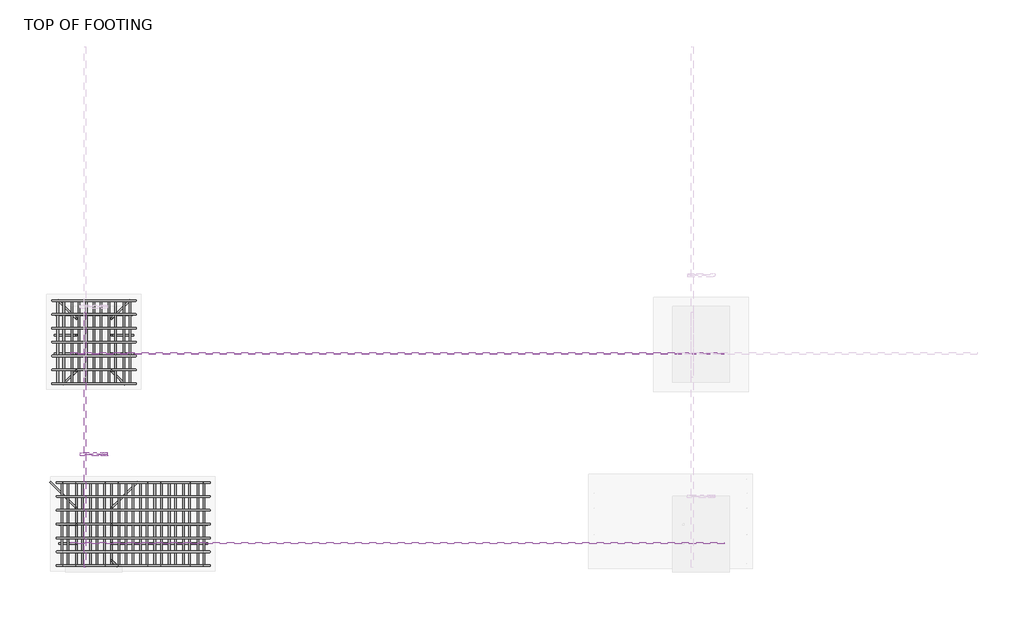
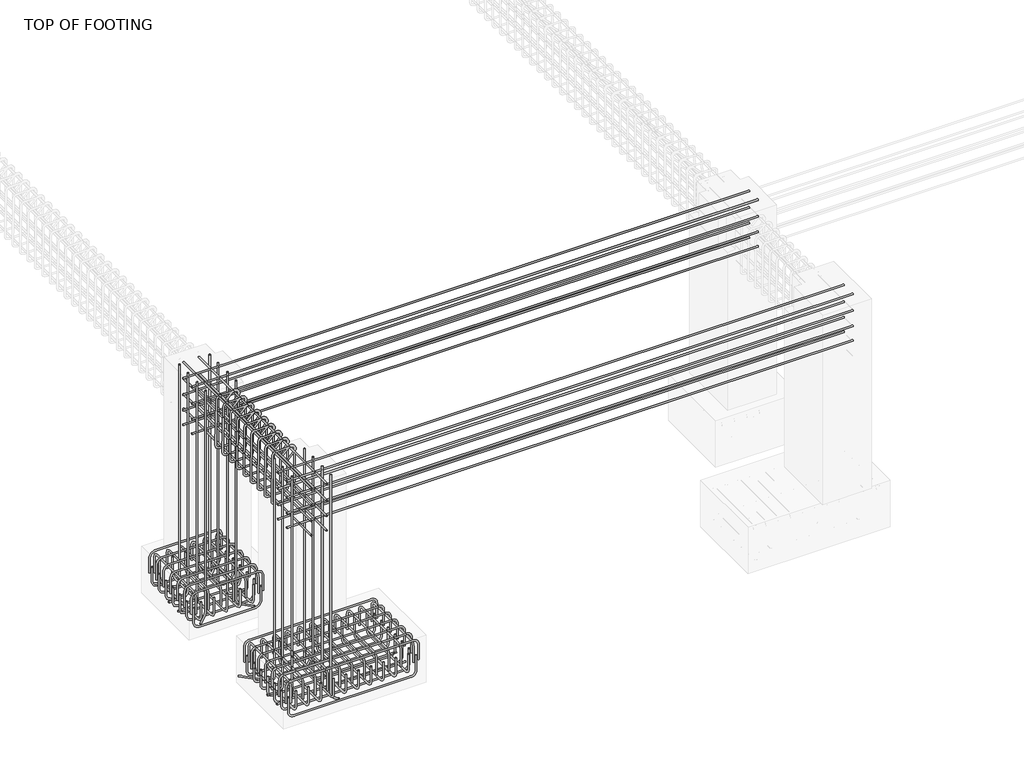
# One storey, part 2 of 8: 32 reinforcing bars.
"""IFC4 building model written with IfcOpenShell, lengths in millimetres."""

from ifc_helpers import new_model, si_unit, point, frame, origin, place, context, project, spatial, polyline, circle_curve, trimmed, segment, composite_curve, source, transform, mapped, element, save
from ifc_brep_helpers import swept_disk

model = new_model("IFC4")

# Units and contexts
model_context = context("Model", 3, world=origin())
ifc_project = project(units=[si_unit("LENGTHUNIT", "METRE", prefix="MILLI")], contexts=[model_context])

# Site, building, storey
site = spatial("IfcSite", under=ifc_project)
building = spatial("IfcBuilding", under=site)
storey = spatial("IfcBuildingStorey", under=building, Name="TOP OF FOOTING", Elevation=-1828.8)

# Reinforcing bars
placement = place(None, origin())
reinforcing_bar_shape = source(origin(), model_context, "Body", "SolidModel", [
    swept_disk(composite_curve([segment(polyline([(-6195.5877818, -134.3579757, -2021.245224), (-6195.5877818, -134.3579757, -2168.545224)]), True, "CONTINUOUS"), segment(trimmed(circle_curve(frame((-6241.9377818, -134.3579757, -2168.545224), z_axis=(0.0, 1.0, 0.0), x_axis=(46.350000000000364, 0.0, 0.0)), 46.35), [point((-6195.5877818, -134.3579757, -2168.545224))], [point((-6241.9377818, -134.3579757, -2214.895224))], True, "CARTESIAN"), True, "CONTINUOUS"), segment(polyline([(-6241.9377818, -134.3579757, -2214.895224), (-6762.8758647, -134.3579757, -2214.895224)]), True, "CONTINUOUS"), segment(trimmed(circle_curve(frame((-6762.8758647, -134.3579757, -2168.545224), z_axis=(0.0, 1.0, 0.0), x_axis=(0.0, 0.0, -46.34999999999991)), 46.35), [point((-6762.8758647, -134.3579757, -2214.895224))], [point((-6809.2258647, -134.3579757, -2168.545224))], True, "CARTESIAN"), True, "CONTINUOUS"), segment(polyline([(-6809.2258647, -134.3579757, -2168.545224), (-6809.2258647, -134.3579757, -2021.245224)]), True, "CONTINUOUS")], self_intersect=False), 6.35),
])
element("IfcReinforcingBar", 1, at=placement, inside=storey, context=model_context, shape_type="MappedRepresentation", body=[
    mapped(reinforcing_bar_shape, transform((0.0, 0.0, 0.0), x_axis=(1.0, 0.0, 0.0), y_axis=(0.0, 1.0, 0.0), z_axis=(0.0, 0.0, 1.0))),
    mapped(reinforcing_bar_shape, transform((0.0, -109.55, 0.0), x_axis=(1.0, 0.0, 0.0), y_axis=(0.0, 1.0, 0.0), z_axis=(0.0, 0.0, 1.0))),
    mapped(reinforcing_bar_shape, transform((0.0, -219.1, 0.0), x_axis=(1.0, 0.0, 0.0), y_axis=(0.0, 1.0, 0.0), z_axis=(0.0, 0.0, 1.0))),
    mapped(reinforcing_bar_shape, transform((0.0, -328.65, 0.0), x_axis=(1.0, 0.0, 0.0), y_axis=(0.0, 1.0, 0.0), z_axis=(0.0, 0.0, 1.0))),
    mapped(reinforcing_bar_shape, transform((0.0, -438.2, 0.0), x_axis=(1.0, 0.0, 0.0), y_axis=(0.0, 1.0, 0.0), z_axis=(0.0, 0.0, 1.0))),
    mapped(reinforcing_bar_shape, transform((0.0, -547.75, 0.0), x_axis=(1.0, 0.0, 0.0), y_axis=(0.0, 1.0, 0.0), z_axis=(0.0, 0.0, 1.0))),
    mapped(reinforcing_bar_shape, transform((0.0, -657.3, 0.0), x_axis=(1.0, 0.0, 0.0), y_axis=(0.0, 1.0, 0.0), z_axis=(0.0, 0.0, 1.0))),
])
reinforcing_bar_2_shape = source(origin(), model_context, "Body", "SolidModel", [
    swept_disk(composite_curve([segment(polyline([(-6831.1461367, -134.3579757, -2068.8), (-6831.1461367, -134.3579757, -1921.5)]), True, "CONTINUOUS"), segment(trimmed(circle_curve(frame((-6784.7961367, -134.3579757, -1921.5), z_axis=(0.0, 1.0, 0.0), x_axis=(-46.350000000000364, 0.0, 0.0)), 46.35), [point((-6831.1461367, -134.3579757, -1921.5))], [point((-6784.7961367, -134.3579757, -1875.15))], True, "CARTESIAN"), True, "CONTINUOUS"), segment(polyline([(-6784.7961367, -134.3579757, -1875.15), (-6220.1961367, -134.3579757, -1875.15)]), True, "CONTINUOUS"), segment(trimmed(circle_curve(frame((-6220.1961367, -134.3579757, -1921.5), z_axis=(0.0, 1.0, 0.0), x_axis=(0.0, 0.0, 46.34999999999991)), 46.35), [point((-6220.1961367, -134.3579757, -1875.15))], [point((-6173.8461367, -134.3579757, -1921.5))], True, "CARTESIAN"), True, "CONTINUOUS"), segment(polyline([(-6173.8461367, -134.3579757, -1921.5), (-6173.8461367, -134.3579757, -2068.8)]), True, "CONTINUOUS")], self_intersect=False), 6.35),
])
element("IfcReinforcingBar", 2, at=placement, inside=storey, context=model_context, shape_type="MappedRepresentation", body=[
    mapped(reinforcing_bar_2_shape, transform((0.0, 0.0, 0.0), x_axis=(1.0, 0.0, 0.0), y_axis=(0.0, 1.0, 0.0), z_axis=(0.0, 0.0, 1.0))),
    mapped(reinforcing_bar_2_shape, transform((0.0, -109.55, 0.0), x_axis=(1.0, 0.0, 0.0), y_axis=(0.0, 1.0, 0.0), z_axis=(0.0, 0.0, 1.0))),
    mapped(reinforcing_bar_2_shape, transform((0.0, -219.1, 0.0), x_axis=(1.0, 0.0, 0.0), y_axis=(0.0, 1.0, 0.0), z_axis=(0.0, 0.0, 1.0))),
    mapped(reinforcing_bar_2_shape, transform((0.0, -328.65, 0.0), x_axis=(1.0, 0.0, 0.0), y_axis=(0.0, 1.0, 0.0), z_axis=(0.0, 0.0, 1.0))),
    mapped(reinforcing_bar_2_shape, transform((0.0, -438.2, 0.0), x_axis=(1.0, 0.0, 0.0), y_axis=(0.0, 1.0, 0.0), z_axis=(0.0, 0.0, 1.0))),
    mapped(reinforcing_bar_2_shape, transform((0.0, -547.75, 0.0), x_axis=(1.0, 0.0, 0.0), y_axis=(0.0, 1.0, 0.0), z_axis=(0.0, 0.0, 1.0))),
    mapped(reinforcing_bar_2_shape, transform((0.0, -657.3, 0.0), x_axis=(1.0, 0.0, 0.0), y_axis=(0.0, 1.0, 0.0), z_axis=(0.0, 0.0, 1.0))),
])
reinforcing_bar_3_shape = source(origin(), model_context, "Body", "SolidModel", [
    swept_disk(composite_curve([segment(polyline([(-6219.0253093, -134.3579757, -2080.9203068), (-6219.0253093, -134.3579757, -1933.6203068)]), True, "CONTINUOUS"), segment(trimmed(circle_curve(frame((-6219.0253093, -180.7079757, -1933.6203068), z_axis=(1.0, 0.0, 0.0), x_axis=(0.0, 46.349999999999994, 0.0)), 46.35), [point((-6219.0253093, -134.3579757, -1933.6203068))], [point((-6219.0253093, -180.7079757, -1887.2703068))], True, "CARTESIAN"), True, "CONTINUOUS"), segment(polyline([(-6219.0253093, -180.7079757, -1887.2703068), (-6219.0253093, -745.3079757, -1887.2703068)]), True, "CONTINUOUS"), segment(trimmed(circle_curve(frame((-6219.0253093, -745.3079757, -1933.6203068), z_axis=(1.0, 0.0, 0.0), x_axis=(0.0, 0.0, 46.34999999999991)), 46.35), [point((-6219.0253093, -745.3079757, -1887.2703068))], [point((-6219.0253093, -791.6579757, -1933.6203068))], True, "CARTESIAN"), True, "CONTINUOUS"), segment(polyline([(-6219.0253093, -791.6579757, -1933.6203068), (-6219.0253093, -791.6579757, -2080.9203068)]), True, "CONTINUOUS")], self_intersect=False), 6.35),
])
element("IfcReinforcingBar", 3, at=placement, inside=storey, context=model_context, shape_type="MappedRepresentation", body=[
    mapped(reinforcing_bar_3_shape, transform((0.0, 0.0, 0.0), x_axis=(1.0, 0.0, 0.0), y_axis=(0.0, 1.0, 0.0), z_axis=(0.0, 0.0, 1.0))),
    mapped(reinforcing_bar_3_shape, transform((-113.9683653, 0.0, 0.0), x_axis=(1.0, 0.0, 0.0), y_axis=(0.0, 1.0, 0.0), z_axis=(0.0, 0.0, 1.0))),
    mapped(reinforcing_bar_3_shape, transform((-227.9367307, 0.0, 0.0), x_axis=(1.0, 0.0, 0.0), y_axis=(0.0, 1.0, 0.0), z_axis=(0.0, 0.0, 1.0))),
    mapped(reinforcing_bar_3_shape, transform((-341.905096, 0.0, 0.0), x_axis=(1.0, 0.0, 0.0), y_axis=(0.0, 1.0, 0.0), z_axis=(0.0, 0.0, 1.0))),
    mapped(reinforcing_bar_3_shape, transform((-455.8734613, 0.0, 0.0), x_axis=(1.0, 0.0, 0.0), y_axis=(0.0, 1.0, 0.0), z_axis=(0.0, 0.0, 1.0))),
    mapped(reinforcing_bar_3_shape, transform((-569.8418267, 0.0, 0.0), x_axis=(1.0, 0.0, 0.0), y_axis=(0.0, 1.0, 0.0), z_axis=(0.0, 0.0, 1.0))),
])
reinforcing_bar_4_shape = source(origin(), model_context, "Body", "SolidModel", [
    swept_disk(composite_curve([segment(polyline([(-6741.3656272, -134.3579757, -1984.9681267), (-6741.3656272, -134.3579757, -2132.2681267)]), True, "CONTINUOUS"), segment(trimmed(circle_curve(frame((-6741.3656272, -180.7079757, -2132.2681267), z_axis=(-1.0, 0.0, 0.0), x_axis=(0.0, 46.349999999999994, 0.0)), 46.35), [point((-6741.3656272, -134.3579757, -2132.2681267))], [point((-6741.3656272, -180.7079757, -2178.6181267))], True, "CARTESIAN"), True, "CONTINUOUS"), segment(polyline([(-6741.3656272, -180.7079757, -2178.6181267), (-6741.3656272, -745.3079757, -2178.6181267)]), True, "CONTINUOUS"), segment(trimmed(circle_curve(frame((-6741.3656272, -745.3079757, -2132.2681267), z_axis=(-1.0, 0.0, 0.0), x_axis=(0.0, 0.0, -46.350000000000364)), 46.35), [point((-6741.3656272, -745.3079757, -2178.6181267))], [point((-6741.3656272, -791.6579757, -2132.2681267))], True, "CARTESIAN"), True, "CONTINUOUS"), segment(polyline([(-6741.3656272, -791.6579757, -2132.2681267), (-6741.3656272, -791.6579757, -1984.9681267)]), True, "CONTINUOUS")], self_intersect=False), 6.35),
])
element("IfcReinforcingBar", 4, at=placement, inside=storey, context=model_context, shape_type="MappedRepresentation", body=[
    mapped(reinforcing_bar_4_shape, transform((0.0, 0.0, 0.0), x_axis=(1.0, 0.0, 0.0), y_axis=(0.0, 1.0, 0.0), z_axis=(0.0, 0.0, 1.0))),
    mapped(reinforcing_bar_4_shape, transform((119.2770606, 0.0, 0.0), x_axis=(1.0, 0.0, 0.0), y_axis=(0.0, 1.0, 0.0), z_axis=(0.0, 0.0, 1.0))),
    mapped(reinforcing_bar_4_shape, transform((238.5541211, 0.0, 0.0), x_axis=(1.0, 0.0, 0.0), y_axis=(0.0, 1.0, 0.0), z_axis=(0.0, 0.0, 1.0))),
    mapped(reinforcing_bar_4_shape, transform((357.8311817, 0.0, 0.0), x_axis=(1.0, 0.0, 0.0), y_axis=(0.0, 1.0, 0.0), z_axis=(0.0, 0.0, 1.0))),
    mapped(reinforcing_bar_4_shape, transform((477.1082423, 0.0, 0.0), x_axis=(1.0, 0.0, 0.0), y_axis=(0.0, 1.0, 0.0), z_axis=(0.0, 0.0, 1.0))),
])
reinforcing_bar_5_shape = source(origin(), model_context, "Body", "SolidModel", [
    swept_disk(composite_curve([segment(polyline([(-5610.5877818, -1574.3579757, -2021.245224), (-5610.5877818, -1574.3579757, -2168.545224)]), True, "CONTINUOUS"), segment(trimmed(circle_curve(frame((-5656.9377818, -1574.3579757, -2168.545224), z_axis=(0.0, 1.0, 0.0), x_axis=(46.350000000000364, 0.0, 0.0)), 46.35), [point((-5610.5877818, -1574.3579757, -2168.545224))], [point((-5656.9377818, -1574.3579757, -2214.895224))], True, "CARTESIAN"), True, "CONTINUOUS"), segment(polyline([(-5656.9377818, -1574.3579757, -2214.895224), (-6727.8758647, -1574.3579757, -2214.895224)]), True, "CONTINUOUS"), segment(trimmed(circle_curve(frame((-6727.8758647, -1574.3579757, -2168.545224), z_axis=(0.0, 1.0, 0.0), x_axis=(0.0, 0.0, -46.34999999999991)), 46.35), [point((-6727.8758647, -1574.3579757, -2214.895224))], [point((-6774.2258647, -1574.3579757, -2168.545224))], True, "CARTESIAN"), True, "CONTINUOUS"), segment(polyline([(-6774.2258647, -1574.3579757, -2168.545224), (-6774.2258647, -1574.3579757, -2021.245224)]), True, "CONTINUOUS")], self_intersect=False), 6.35),
])
element("IfcReinforcingBar", 5, at=placement, inside=storey, context=model_context, shape_type="MappedRepresentation", body=[
    mapped(reinforcing_bar_5_shape, transform((0.0, 0.0, 0.0), x_axis=(1.0, 0.0, 0.0), y_axis=(0.0, 1.0, 0.0), z_axis=(0.0, 0.0, 1.0))),
    mapped(reinforcing_bar_5_shape, transform((0.0, -109.55, 0.0), x_axis=(1.0, 0.0, 0.0), y_axis=(0.0, 1.0, 0.0), z_axis=(0.0, 0.0, 1.0))),
    mapped(reinforcing_bar_5_shape, transform((0.0, -219.1, 0.0), x_axis=(1.0, 0.0, 0.0), y_axis=(0.0, 1.0, 0.0), z_axis=(0.0, 0.0, 1.0))),
    mapped(reinforcing_bar_5_shape, transform((0.0, -328.65, 0.0), x_axis=(1.0, 0.0, 0.0), y_axis=(0.0, 1.0, 0.0), z_axis=(0.0, 0.0, 1.0))),
    mapped(reinforcing_bar_5_shape, transform((0.0, -438.2, 0.0), x_axis=(1.0, 0.0, 0.0), y_axis=(0.0, 1.0, 0.0), z_axis=(0.0, 0.0, 1.0))),
    mapped(reinforcing_bar_5_shape, transform((0.0, -547.75, 0.0), x_axis=(1.0, 0.0, 0.0), y_axis=(0.0, 1.0, 0.0), z_axis=(0.0, 0.0, 1.0))),
    mapped(reinforcing_bar_5_shape, transform((0.0, -657.3, 0.0), x_axis=(1.0, 0.0, 0.0), y_axis=(0.0, 1.0, 0.0), z_axis=(0.0, 0.0, 1.0))),
])
reinforcing_bar_6_shape = source(origin(), model_context, "Body", "SolidModel", [
    swept_disk(composite_curve([segment(polyline([(-6796.1461367, -1574.3579757, -2068.8), (-6796.1461367, -1574.3579757, -1921.5)]), True, "CONTINUOUS"), segment(trimmed(circle_curve(frame((-6749.7961367, -1574.3579757, -1921.5), z_axis=(0.0, 1.0, 0.0), x_axis=(-46.350000000000364, 0.0, 0.0)), 46.35), [point((-6796.1461367, -1574.3579757, -1921.5))], [point((-6749.7961367, -1574.3579757, -1875.15))], True, "CARTESIAN"), True, "CONTINUOUS"), segment(polyline([(-6749.7961367, -1574.3579757, -1875.15), (-5635.1961367, -1574.3579757, -1875.15)]), True, "CONTINUOUS"), segment(trimmed(circle_curve(frame((-5635.1961367, -1574.3579757, -1921.5), z_axis=(0.0, 1.0, 0.0), x_axis=(0.0, 0.0, 46.34999999999991)), 46.35), [point((-5635.1961367, -1574.3579757, -1875.15))], [point((-5588.8461367, -1574.3579757, -1921.5))], True, "CARTESIAN"), True, "CONTINUOUS"), segment(polyline([(-5588.8461367, -1574.3579757, -1921.5), (-5588.8461367, -1574.3579757, -2068.8)]), True, "CONTINUOUS")], self_intersect=False), 6.35),
])
element("IfcReinforcingBar", 6, at=placement, inside=storey, context=model_context, shape_type="MappedRepresentation", body=[
    mapped(reinforcing_bar_6_shape, transform((0.0, 0.0, 0.0), x_axis=(1.0, 0.0, 0.0), y_axis=(0.0, 1.0, 0.0), z_axis=(0.0, 0.0, 1.0))),
    mapped(reinforcing_bar_6_shape, transform((0.0, -109.55, 0.0), x_axis=(1.0, 0.0, 0.0), y_axis=(0.0, 1.0, 0.0), z_axis=(0.0, 0.0, 1.0))),
    mapped(reinforcing_bar_6_shape, transform((0.0, -219.1, 0.0), x_axis=(1.0, 0.0, 0.0), y_axis=(0.0, 1.0, 0.0), z_axis=(0.0, 0.0, 1.0))),
    mapped(reinforcing_bar_6_shape, transform((0.0, -328.65, 0.0), x_axis=(1.0, 0.0, 0.0), y_axis=(0.0, 1.0, 0.0), z_axis=(0.0, 0.0, 1.0))),
    mapped(reinforcing_bar_6_shape, transform((0.0, -438.2, 0.0), x_axis=(1.0, 0.0, 0.0), y_axis=(0.0, 1.0, 0.0), z_axis=(0.0, 0.0, 1.0))),
    mapped(reinforcing_bar_6_shape, transform((0.0, -547.75, 0.0), x_axis=(1.0, 0.0, 0.0), y_axis=(0.0, 1.0, 0.0), z_axis=(0.0, 0.0, 1.0))),
    mapped(reinforcing_bar_6_shape, transform((0.0, -657.3, 0.0), x_axis=(1.0, 0.0, 0.0), y_axis=(0.0, 1.0, 0.0), z_axis=(0.0, 0.0, 1.0))),
])
reinforcing_bar_7_shape = source(origin(), model_context, "Body", "SolidModel", [
    swept_disk(composite_curve([segment(polyline([(-5634.0253093, -1574.3579757, -2080.9203068), (-5634.0253093, -1574.3579757, -1933.6203068)]), True, "CONTINUOUS"), segment(trimmed(circle_curve(frame((-5634.0253093, -1620.7079757, -1933.6203068), z_axis=(1.0, 0.0, 0.0), x_axis=(0.0, 46.34999999999991, 0.0)), 46.35), [point((-5634.0253093, -1574.3579757, -1933.6203068))], [point((-5634.0253093, -1620.7079757, -1887.2703068))], True, "CARTESIAN"), True, "CONTINUOUS"), segment(polyline([(-5634.0253093, -1620.7079757, -1887.2703068), (-5634.0253093, -2185.3079757, -1887.2703068)]), True, "CONTINUOUS"), segment(trimmed(circle_curve(frame((-5634.0253093, -2185.3079757, -1933.6203068), z_axis=(1.0, 0.0, 0.0), x_axis=(0.0, 0.0, 46.34999999999991)), 46.35), [point((-5634.0253093, -2185.3079757, -1887.2703068))], [point((-5634.0253093, -2231.6579757, -1933.6203068))], True, "CARTESIAN"), True, "CONTINUOUS"), segment(polyline([(-5634.0253093, -2231.6579757, -1933.6203068), (-5634.0253093, -2231.6579757, -2080.9203068)]), True, "CONTINUOUS")], self_intersect=False), 6.35),
])
element("IfcReinforcingBar", 7, at=placement, inside=storey, context=model_context, shape_type="MappedRepresentation", body=[
    mapped(reinforcing_bar_7_shape, transform((0.0, 0.0, 0.0), x_axis=(1.0, 0.0, 0.0), y_axis=(0.0, 1.0, 0.0), z_axis=(0.0, 0.0, 1.0))),
    mapped(reinforcing_bar_7_shape, transform((-111.9841827, 0.0, 0.0), x_axis=(1.0, 0.0, 0.0), y_axis=(0.0, 1.0, 0.0), z_axis=(0.0, 0.0, 1.0))),
    mapped(reinforcing_bar_7_shape, transform((-223.9683653, 0.0, 0.0), x_axis=(1.0, 0.0, 0.0), y_axis=(0.0, 1.0, 0.0), z_axis=(0.0, 0.0, 1.0))),
    mapped(reinforcing_bar_7_shape, transform((-335.952548, 0.0, 0.0), x_axis=(1.0, 0.0, 0.0), y_axis=(0.0, 1.0, 0.0), z_axis=(0.0, 0.0, 1.0))),
    mapped(reinforcing_bar_7_shape, transform((-447.9367307, 0.0, 0.0), x_axis=(1.0, 0.0, 0.0), y_axis=(0.0, 1.0, 0.0), z_axis=(0.0, 0.0, 1.0))),
    mapped(reinforcing_bar_7_shape, transform((-559.9209133, 0.0, 0.0), x_axis=(1.0, 0.0, 0.0), y_axis=(0.0, 1.0, 0.0), z_axis=(0.0, 0.0, 1.0))),
    mapped(reinforcing_bar_7_shape, transform((-671.905096, 0.0, 0.0), x_axis=(1.0, 0.0, 0.0), y_axis=(0.0, 1.0, 0.0), z_axis=(0.0, 0.0, 1.0))),
    mapped(reinforcing_bar_7_shape, transform((-783.8892787, 0.0, 0.0), x_axis=(1.0, 0.0, 0.0), y_axis=(0.0, 1.0, 0.0), z_axis=(0.0, 0.0, 1.0))),
    mapped(reinforcing_bar_7_shape, transform((-895.8734613, 0.0, 0.0), x_axis=(1.0, 0.0, 0.0), y_axis=(0.0, 1.0, 0.0), z_axis=(0.0, 0.0, 1.0))),
    mapped(reinforcing_bar_7_shape, transform((-1007.857644, 0.0, 0.0), x_axis=(1.0, 0.0, 0.0), y_axis=(0.0, 1.0, 0.0), z_axis=(0.0, 0.0, 1.0))),
    mapped(reinforcing_bar_7_shape, transform((-1119.8418267, 0.0, 0.0), x_axis=(1.0, 0.0, 0.0), y_axis=(0.0, 1.0, 0.0), z_axis=(0.0, 0.0, 1.0))),
])
reinforcing_bar_8_shape = source(origin(), model_context, "Body", "SolidModel", [
    swept_disk(composite_curve([segment(polyline([(-6706.3656272, -1574.3579757, -1984.9681267), (-6706.3656272, -1574.3579757, -2132.2681267)]), True, "CONTINUOUS"), segment(trimmed(circle_curve(frame((-6706.3656272, -1620.7079757, -2132.2681267), z_axis=(-1.0, 0.0, 0.0), x_axis=(0.0, 46.34999999999991, 0.0)), 46.35), [point((-6706.3656272, -1574.3579757, -2132.2681267))], [point((-6706.3656272, -1620.7079757, -2178.6181267))], True, "CARTESIAN"), True, "CONTINUOUS"), segment(polyline([(-6706.3656272, -1620.7079757, -2178.6181267), (-6706.3656272, -2185.3079757, -2178.6181267)]), True, "CONTINUOUS"), segment(trimmed(circle_curve(frame((-6706.3656272, -2185.3079757, -2132.2681267), z_axis=(-1.0, 0.0, 0.0), x_axis=(0.0, 0.0, -46.350000000000364)), 46.35), [point((-6706.3656272, -2185.3079757, -2178.6181267))], [point((-6706.3656272, -2231.6579757, -2132.2681267))], True, "CARTESIAN"), True, "CONTINUOUS"), segment(polyline([(-6706.3656272, -2231.6579757, -2132.2681267), (-6706.3656272, -2231.6579757, -1984.9681267)]), True, "CONTINUOUS")], self_intersect=False), 6.35),
])
element("IfcReinforcingBar", 8, at=placement, inside=storey, context=model_context, shape_type="MappedRepresentation", body=[
    mapped(reinforcing_bar_8_shape, transform((0.0, 0.0, 0.0), x_axis=(1.0, 0.0, 0.0), y_axis=(0.0, 1.0, 0.0), z_axis=(0.0, 0.0, 1.0))),
    mapped(reinforcing_bar_8_shape, transform((114.123138, 0.0, 0.0), x_axis=(1.0, 0.0, 0.0), y_axis=(0.0, 1.0, 0.0), z_axis=(0.0, 0.0, 1.0))),
    mapped(reinforcing_bar_8_shape, transform((228.2462761, 0.0, 0.0), x_axis=(1.0, 0.0, 0.0), y_axis=(0.0, 1.0, 0.0), z_axis=(0.0, 0.0, 1.0))),
    mapped(reinforcing_bar_8_shape, transform((342.3694141, 0.0, 0.0), x_axis=(1.0, 0.0, 0.0), y_axis=(0.0, 1.0, 0.0), z_axis=(0.0, 0.0, 1.0))),
    mapped(reinforcing_bar_8_shape, transform((456.4925521, 0.0, 0.0), x_axis=(1.0, 0.0, 0.0), y_axis=(0.0, 1.0, 0.0), z_axis=(0.0, 0.0, 1.0))),
    mapped(reinforcing_bar_8_shape, transform((570.6156901, 0.0, 0.0), x_axis=(1.0, 0.0, 0.0), y_axis=(0.0, 1.0, 0.0), z_axis=(0.0, 0.0, 1.0))),
    mapped(reinforcing_bar_8_shape, transform((684.7388282, 0.0, 0.0), x_axis=(1.0, 0.0, 0.0), y_axis=(0.0, 1.0, 0.0), z_axis=(0.0, 0.0, 1.0))),
    mapped(reinforcing_bar_8_shape, transform((798.8619662, 0.0, 0.0), x_axis=(1.0, 0.0, 0.0), y_axis=(0.0, 1.0, 0.0), z_axis=(0.0, 0.0, 1.0))),
    mapped(reinforcing_bar_8_shape, transform((912.9851042, 0.0, 0.0), x_axis=(1.0, 0.0, 0.0), y_axis=(0.0, 1.0, 0.0), z_axis=(0.0, 0.0, 1.0))),
    mapped(reinforcing_bar_8_shape, transform((1027.1082423, 0.0, 0.0), x_axis=(1.0, 0.0, 0.0), y_axis=(0.0, 1.0, 0.0), z_axis=(0.0, 0.0, 1.0))),
])
reinforcing_bar_9_shape = source(origin(), model_context, "Body", "SolidModel", [
    swept_disk(composite_curve([segment(polyline([(-6815.4438347, -407.8655692, -2192.6897268), (-6687.1151723, -407.8655692, -2192.6897268)]), True, "CONTINUOUS"), segment(trimmed(circle_curve(frame((-6687.1151723, -407.8655692, -2146.3397268), z_axis=(0.0, -1.0, 0.0), x_axis=(0.0, 0.0, -46.34999999999991)), 46.35), [point((-6687.1151723, -407.8655692, -2192.6897268))], [point((-6640.7651723, -407.8655692, -2146.3397268))], True, "CARTESIAN"), True, "CONTINUOUS"), segment(polyline([(-6640.7651723, -407.8655692, -2146.3397268), (-6640.7651723, -407.8655692, -40.0)]), True, "CONTINUOUS")], self_intersect=False), 6.35),
])
element("IfcReinforcingBar", 9, at=placement, inside=storey, context=model_context, shape_type="MappedRepresentation", body=[
    mapped(reinforcing_bar_9_shape, transform((0.0, 0.0, 0.0), x_axis=(1.0, 0.0, 0.0), y_axis=(0.0, 1.0, 0.0), z_axis=(0.0, 0.0, 1.0))),
    mapped(reinforcing_bar_9_shape, transform((0.0, -147.7903727, 0.0), x_axis=(1.0, 0.0, 0.0), y_axis=(0.0, 1.0, 0.0), z_axis=(0.0, 0.0, 1.0))),
])
element("IfcReinforcingBar", 10, at=placement, inside=storey, context=model_context, shape_type="SolidModel", body=[
    swept_disk(composite_curve([segment(polyline([(-6748.0144002, -797.3699065, -2192.6897268), (-6673.5395717, -722.8950779, -2192.6897268)]), True, "CONTINUOUS"), segment(trimmed(circle_curve(frame((-6673.5395717, -722.8950779, -2146.3397268), z_axis=(0.7071067811865476, -0.7071067811865475, 0.0), x_axis=(0.0, 0.0, -46.34999999999991)), 46.35), [point((-6673.5395717, -722.8950779, -2192.6897268))], [point((-6640.7651723, -690.1206786, -2146.3397268))], True, "CARTESIAN"), True, "CONTINUOUS"), segment(polyline([(-6640.7651723, -690.1206786, -2146.3397268), (-6640.7651723, -690.1206786, -40.0)]), True, "CONTINUOUS")], self_intersect=False), 6.35),
])
element("IfcReinforcingBar", 11, at=placement, inside=storey, context=model_context, shape_type="SolidModel", body=[
    swept_disk(composite_curve([segment(polyline([(-6256.9778732, -797.3699065, -2192.6897268), (-6331.4527018, -722.8950779, -2192.6897268)]), True, "CONTINUOUS"), segment(trimmed(circle_curve(frame((-6331.4527018, -722.8950779, -2146.3397268), z_axis=(0.7071067811865754, 0.7071067811865197, 0.0), x_axis=(0.0, 0.0, -46.34999999999991)), 46.35), [point((-6331.4527018, -722.8950779, -2192.6897268))], [point((-6364.2271011, -690.1206786, -2146.3397268))], True, "CARTESIAN"), True, "CONTINUOUS"), segment(polyline([(-6364.2271011, -690.1206786, -2146.3397268), (-6364.2271011, -690.1206786, -40.0)]), True, "CONTINUOUS")], self_intersect=False), 6.35),
])
element("IfcReinforcingBar", 12, at=placement, inside=storey, context=model_context, shape_type="SolidModel", body=[
    swept_disk(composite_curve([segment(polyline([(-6788.0144002, -128.646045, -2192.6897268), (-6673.5395717, -243.1208736, -2192.6897268)]), True, "CONTINUOUS"), segment(trimmed(circle_curve(frame((-6673.5395717, -243.1208736, -2146.3397268), z_axis=(-0.7071067811865389, -0.7071067811865562, 0.0), x_axis=(0.0, 0.0, -46.34999999999991)), 46.35), [point((-6673.5395717, -243.1208736, -2192.6897268))], [point((-6640.7651723, -275.8952729, -2146.3397268))], True, "CARTESIAN"), True, "CONTINUOUS"), segment(polyline([(-6640.7651723, -275.8952729, -2146.3397268), (-6640.7651723, -275.8952729, -40.0)]), True, "CONTINUOUS")], self_intersect=False), 6.35),
])
element("IfcReinforcingBar", 13, at=placement, inside=storey, context=model_context, shape_type="SolidModel", body=[
    swept_disk(composite_curve([segment(polyline([(-6216.9778732, -128.646045, -2192.6897268), (-6331.4527018, -243.1208736, -2192.6897268)]), True, "CONTINUOUS"), segment(trimmed(circle_curve(frame((-6331.4527018, -243.1208736, -2146.3397268), z_axis=(-0.707106781186584, 0.707106781186511, 0.0), x_axis=(0.0, 0.0, -46.34999999999991)), 46.35), [point((-6331.4527018, -243.1208736, -2192.6897268))], [point((-6364.2271011, -275.8952729, -2146.3397268))], True, "CARTESIAN"), True, "CONTINUOUS"), segment(polyline([(-6364.2271011, -275.8952729, -2146.3397268), (-6364.2271011, -275.8952729, -40.0)]), True, "CONTINUOUS")], self_intersect=False), 6.35),
])
reinforcing_bar_10_shape = source(origin(), model_context, "Body", "SolidModel", [
    swept_disk(composite_curve([segment(polyline([(-6189.5484388, -407.8655692, -2192.6897268), (-6317.8771011, -407.8655692, -2192.6897268)]), True, "CONTINUOUS"), segment(trimmed(circle_curve(frame((-6317.8771011, -407.8655692, -2146.3397268), z_axis=(0.0, 1.0, 0.0), x_axis=(0.0, 0.0, -46.34999999999991)), 46.35), [point((-6317.8771011, -407.8655692, -2192.6897268))], [point((-6364.2271011, -407.8655692, -2146.3397268))], True, "CARTESIAN"), True, "CONTINUOUS"), segment(polyline([(-6364.2271011, -407.8655692, -2146.3397268), (-6364.2271011, -407.8655692, -40.0)]), True, "CONTINUOUS")], self_intersect=False), 6.35),
])
element("IfcReinforcingBar", 14, at=placement, inside=storey, context=model_context, shape_type="MappedRepresentation", body=[
    mapped(reinforcing_bar_10_shape, transform((0.0, 0.0, 0.0), x_axis=(1.0, 0.0, 0.0), y_axis=(0.0, 1.0, 0.0), z_axis=(0.0, 0.0, 1.0))),
    mapped(reinforcing_bar_10_shape, transform((0.0, -147.7903727, 0.0), x_axis=(1.0, 0.0, 0.0), y_axis=(0.0, 1.0, 0.0), z_axis=(0.0, 0.0, 1.0))),
])
reinforcing_bar_11_shape = source(origin(), model_context, "Body", "SolidModel", [
    swept_disk(composite_curve([segment(polyline([(-6780.4438347, -1907.8655692, -2192.6897268), (-6687.1151723, -1907.8655692, -2192.6897268)]), True, "CONTINUOUS"), segment(trimmed(circle_curve(frame((-6687.1151723, -1907.8655692, -2146.3397268), z_axis=(0.0, -1.0, 0.0), x_axis=(0.0, 0.0, -46.34999999999991)), 46.35), [point((-6687.1151723, -1907.8655692, -2192.6897268))], [point((-6640.7651723, -1907.8655692, -2146.3397268))], True, "CARTESIAN"), True, "CONTINUOUS"), segment(polyline([(-6640.7651723, -1907.8655692, -2146.3397268), (-6640.7651723, -1907.8655692, -40.0)]), True, "CONTINUOUS")], self_intersect=False), 6.35),
])
element("IfcReinforcingBar", 15, at=placement, inside=storey, context=model_context, shape_type="MappedRepresentation", body=[
    mapped(reinforcing_bar_11_shape, transform((0.0, 0.0, 0.0), x_axis=(1.0, 0.0, 0.0), y_axis=(0.0, 1.0, 0.0), z_axis=(0.0, 0.0, 1.0))),
    mapped(reinforcing_bar_11_shape, transform((0.0, -147.7903727, 0.0), x_axis=(1.0, 0.0, 0.0), y_axis=(0.0, 1.0, 0.0), z_axis=(0.0, 0.0, 1.0))),
])
element("IfcReinforcingBar", 16, at=placement, inside=storey, context=model_context, shape_type="SolidModel", body=[
    swept_disk(composite_curve([segment(polyline([(-6316.9778732, -2237.3699065, -2192.6897268), (-6331.4527018, -2222.8950779, -2192.6897268)]), True, "CONTINUOUS"), segment(trimmed(circle_curve(frame((-6331.4527018, -2222.8950779, -2146.3397268), z_axis=(0.7071067811865754, 0.7071067811865197, 0.0), x_axis=(0.0, 0.0, -46.34999999999991)), 46.35), [point((-6331.4527018, -2222.8950779, -2192.6897268))], [point((-6364.2271011, -2190.1206786, -2146.3397268))], True, "CARTESIAN"), True, "CONTINUOUS"), segment(polyline([(-6364.2271011, -2190.1206786, -2146.3397268), (-6364.2271011, -2190.1206786, -40.0)]), True, "CONTINUOUS")], self_intersect=False), 6.35),
])
element("IfcReinforcingBar", 17, at=placement, inside=storey, context=model_context, shape_type="SolidModel", body=[
    swept_disk(composite_curve([segment(polyline([(-6848.0144002, -1568.646045, -2192.6897268), (-6673.5395717, -1743.1208736, -2192.6897268)]), True, "CONTINUOUS"), segment(trimmed(circle_curve(frame((-6673.5395717, -1743.1208736, -2146.3397268), z_axis=(-0.707106781186539, -0.7071067811865561, 0.0), x_axis=(0.0, 0.0, -46.34999999999991)), 46.35), [point((-6673.5395717, -1743.1208736, -2192.6897268))], [point((-6640.7651723, -1775.8952729, -2146.3397268))], True, "CARTESIAN"), True, "CONTINUOUS"), segment(polyline([(-6640.7651723, -1775.8952729, -2146.3397268), (-6640.7651723, -1775.8952729, -40.0)]), True, "CONTINUOUS")], self_intersect=False), 6.35),
])
element("IfcReinforcingBar", 18, at=placement, inside=storey, context=model_context, shape_type="SolidModel", body=[
    swept_disk(composite_curve([segment(polyline([(-6156.9778732, -1568.646045, -2192.6897268), (-6331.4527018, -1743.1208736, -2192.6897268)]), True, "CONTINUOUS"), segment(trimmed(circle_curve(frame((-6331.4527018, -1743.1208736, -2146.3397268), z_axis=(-0.707106781186584, 0.7071067811865112, 0.0), x_axis=(0.0, 0.0, -46.34999999999991)), 46.35), [point((-6331.4527018, -1743.1208736, -2192.6897268))], [point((-6364.2271011, -1775.8952729, -2146.3397268))], True, "CARTESIAN"), True, "CONTINUOUS"), segment(polyline([(-6364.2271011, -1775.8952729, -2146.3397268), (-6364.2271011, -1775.8952729, -40.0)]), True, "CONTINUOUS")], self_intersect=False), 6.35),
])
reinforcing_bar_12_shape = source(origin(), model_context, "Body", "SolidModel", [
    swept_disk(composite_curve([segment(polyline([(-5604.5484388, -1907.8655692, -2192.6897268), (-6317.8771011, -1907.8655692, -2192.6897268)]), True, "CONTINUOUS"), segment(trimmed(circle_curve(frame((-6317.8771011, -1907.8655692, -2146.3397268), z_axis=(0.0, 1.0, 0.0), x_axis=(0.0, 0.0, -46.34999999999991)), 46.35), [point((-6317.8771011, -1907.8655692, -2192.6897268))], [point((-6364.2271011, -1907.8655692, -2146.3397268))], True, "CARTESIAN"), True, "CONTINUOUS"), segment(polyline([(-6364.2271011, -1907.8655692, -2146.3397268), (-6364.2271011, -1907.8655692, -40.0)]), True, "CONTINUOUS")], self_intersect=False), 6.35),
])
element("IfcReinforcingBar", 19, at=placement, inside=storey, context=model_context, shape_type="MappedRepresentation", body=[
    mapped(reinforcing_bar_12_shape, transform((0.0, 0.0, 0.0), x_axis=(1.0, 0.0, 0.0), y_axis=(0.0, 1.0, 0.0), z_axis=(0.0, 0.0, 1.0))),
    mapped(reinforcing_bar_12_shape, transform((0.0, -147.7903727, 0.0), x_axis=(1.0, 0.0, 0.0), y_axis=(0.0, 1.0, 0.0), z_axis=(0.0, 0.0, 1.0))),
])
reinforcing_bar_13_shape = source(origin(), model_context, "Body", "SolidModel", [
    swept_disk(composite_curve([segment(polyline([(-6508.1074973, -1676.6579757, -111.2757654), (-6452.3639343, -1676.6579757, -55.5322024)]), True, "CONTINUOUS"), segment(trimmed(circle_curve(frame((-6430.1961367, -1676.6579757, -77.7), z_axis=(0.0, 1.0, 0.0), x_axis=(-22.167797600000085, 0.0, 22.1677976)), 31.35), [point((-6452.3639343, -1676.6579757, -55.5322024))], [point((-6398.8461367, -1676.6579757, -77.7))], True, "CARTESIAN"), True, "CONTINUOUS"), segment(polyline([(-6398.8461367, -1676.6579757, -77.7), (-6398.8461367, -1676.6579757, -522.3)]), True, "CONTINUOUS"), segment(trimmed(circle_curve(frame((-6430.1961367, -1676.6579757, -522.3), z_axis=(0.0, 1.0, 0.0), x_axis=(31.350000000000364, 0.0, 0.0)), 31.35), [point((-6398.8461367, -1676.6579757, -522.3))], [point((-6430.1961367, -1676.6579757, -553.65))], True, "CARTESIAN"), True, "CONTINUOUS"), segment(polyline([(-6430.1961367, -1676.6579757, -553.65), (-6574.7961367, -1676.6579757, -553.65)]), True, "CONTINUOUS"), segment(trimmed(circle_curve(frame((-6574.7961367, -1677.4425614, -522.3098193), z_axis=(0.0, 0.9996867842138424, 0.025026655153786322), x_axis=(0.0, 0.7845856999999796, -31.34018070000002)), 31.35), [point((-6574.7961367, -1676.6579757, -553.65))], [point((-6606.1461367, -1677.4425614, -522.3098193))], True, "CARTESIAN"), True, "CONTINUOUS"), segment(polyline([(-6606.1461367, -1677.4425614, -522.3098193), (-6606.1461367, -1688.5733901, -77.6901807)]), True, "CONTINUOUS"), segment(trimmed(circle_curve(frame((-6574.7961367, -1688.5733901, -77.6901807), z_axis=(0.0, 0.9996867842138424, 0.025026655153786322), x_axis=(-31.350000000000364, 0.0, 0.0)), 31.35), [point((-6606.1461367, -1688.5733901, -77.6901807))], [point((-6574.7961367, -1689.3579757, -46.35))], True, "CARTESIAN"), True, "CONTINUOUS"), segment(polyline([(-6574.7961367, -1689.3579757, -46.35), (-6430.1961367, -1689.3579757, -46.35)]), True, "CONTINUOUS"), segment(trimmed(circle_curve(frame((-6430.1961367, -1689.3579757, -77.7), z_axis=(0.0, 1.0, 0.0), x_axis=(0.0, 0.0, 31.35)), 31.35), [point((-6430.1961367, -1689.3579757, -46.35))], [point((-6408.0283391, -1689.3579757, -99.8677976))], True, "CARTESIAN"), True, "CONTINUOUS"), segment(polyline([(-6408.0283391, -1689.3579757, -99.8677976), (-6463.7719021, -1689.3579757, -155.6113605)]), True, "CONTINUOUS")], self_intersect=False), 6.35),
])
element("IfcReinforcingBar", 20, at=placement, inside=storey, context=model_context, shape_type="MappedRepresentation", body=[
    mapped(reinforcing_bar_13_shape, transform((0.0, 0.0, 0.0), x_axis=(1.0, 0.0, 0.0), y_axis=(0.0, 1.0, 0.0), z_axis=(0.0, 0.0, 1.0))),
    mapped(reinforcing_bar_13_shape, transform((0.0, 110.9125, 0.0), x_axis=(1.0, 0.0, 0.0), y_axis=(0.0, 1.0, 0.0), z_axis=(0.0, 0.0, 1.0))),
    mapped(reinforcing_bar_13_shape, transform((0.0, 221.825, 0.0), x_axis=(1.0, 0.0, 0.0), y_axis=(0.0, 1.0, 0.0), z_axis=(0.0, 0.0, 1.0))),
    mapped(reinforcing_bar_13_shape, transform((0.0, 332.7375, 0.0), x_axis=(1.0, 0.0, 0.0), y_axis=(0.0, 1.0, 0.0), z_axis=(0.0, 0.0, 1.0))),
    mapped(reinforcing_bar_13_shape, transform((0.0, 443.65, 0.0), x_axis=(1.0, 0.0, 0.0), y_axis=(0.0, 1.0, 0.0), z_axis=(0.0, 0.0, 1.0))),
    mapped(reinforcing_bar_13_shape, transform((0.0, 554.5625, 0.0), x_axis=(1.0, 0.0, 0.0), y_axis=(0.0, 1.0, 0.0), z_axis=(0.0, 0.0, 1.0))),
    mapped(reinforcing_bar_13_shape, transform((0.0, 665.475, 0.0), x_axis=(1.0, 0.0, 0.0), y_axis=(0.0, 1.0, 0.0), z_axis=(0.0, 0.0, 1.0))),
    mapped(reinforcing_bar_13_shape, transform((0.0, 776.3875, 0.0), x_axis=(1.0, 0.0, 0.0), y_axis=(0.0, 1.0, 0.0), z_axis=(0.0, 0.0, 1.0))),
    mapped(reinforcing_bar_13_shape, transform((0.0, 887.3, 0.0), x_axis=(1.0, 0.0, 0.0), y_axis=(0.0, 1.0, 0.0), z_axis=(0.0, 0.0, 1.0))),
])
reinforcing_bar_14_shape = source(origin(), model_context, "Body", "SolidModel", [
    swept_disk(composite_curve([segment(polyline([(-6572.1179081, -2243.0079757, -72.7), (-6572.1179081, -223.0079757, -72.7)]), True, "CONTINUOUS")], self_intersect=False), 6.35),
])
element("IfcReinforcingBar", 21, at=placement, inside=storey, context=model_context, shape_type="MappedRepresentation", body=[
    mapped(reinforcing_bar_14_shape, transform((0.0, 0.0, 0.0), x_axis=(1.0, 0.0, 0.0), y_axis=(0.0, 1.0, 0.0), z_axis=(0.0, 0.0, 1.0))),
    mapped(reinforcing_bar_14_shape, transform((139.7429418, 0.0, 0.0), x_axis=(1.0, 0.0, 0.0), y_axis=(0.0, 1.0, 0.0), z_axis=(0.0, 0.0, 1.0))),
])
reinforcing_bar_15_shape = source(origin(), model_context, "Body", "SolidModel", [
    swept_disk(composite_curve([segment(polyline([(-6572.1179081, -2243.0079757, -522.7), (-6572.1179081, -223.0079757, -522.7)]), True, "CONTINUOUS")], self_intersect=False), 6.35),
])
element("IfcReinforcingBar", 22, at=placement, inside=storey, context=model_context, shape_type="MappedRepresentation", body=[
    mapped(reinforcing_bar_15_shape, transform((0.0, 0.0, 0.0), x_axis=(1.0, 0.0, 0.0), y_axis=(0.0, 1.0, 0.0), z_axis=(0.0, 0.0, 1.0))),
    mapped(reinforcing_bar_15_shape, transform((139.7429418, 0.0, 0.0), x_axis=(1.0, 0.0, 0.0), y_axis=(0.0, 1.0, 0.0), z_axis=(0.0, 0.0, 1.0))),
])
reinforcing_bar_16_shape = source(origin(), model_context, "Body", "SolidModel", [
    swept_disk(composite_curve([segment(polyline([(-6572.1179081, -2243.0079757, -382.7), (-6572.1179081, -223.0079757, -382.7)]), True, "CONTINUOUS")], self_intersect=False), 6.35),
])
element("IfcReinforcingBar", 23, at=placement, inside=storey, context=model_context, shape_type="MappedRepresentation", body=[
    mapped(reinforcing_bar_16_shape, transform((0.0, 0.0, 0.0), x_axis=(1.0, 0.0, 0.0), y_axis=(0.0, 1.0, 0.0), z_axis=(0.0, 0.0, 1.0))),
    mapped(reinforcing_bar_16_shape, transform((139.7429418, 0.0, 0.0), x_axis=(1.0, 0.0, 0.0), y_axis=(0.0, 1.0, 0.0), z_axis=(0.0, 0.0, 1.0))),
])
reinforcing_bar_17_shape = source(origin(), model_context, "Body", "SolidModel", [
    swept_disk(composite_curve([segment(polyline([(-6572.1179081, -2243.0079757, -232.7), (-6572.1179081, -223.0079757, -232.7)]), True, "CONTINUOUS")], self_intersect=False), 6.35),
])
element("IfcReinforcingBar", 24, at=placement, inside=storey, context=model_context, shape_type="MappedRepresentation", body=[
    mapped(reinforcing_bar_17_shape, transform((0.0, 0.0, 0.0), x_axis=(1.0, 0.0, 0.0), y_axis=(0.0, 1.0, 0.0), z_axis=(0.0, 0.0, 1.0))),
    mapped(reinforcing_bar_17_shape, transform((139.7429418, 0.0, 0.0), x_axis=(1.0, 0.0, 0.0), y_axis=(0.0, 1.0, 0.0), z_axis=(0.0, 0.0, 1.0))),
])
reinforcing_bar_18_shape = source(origin(), model_context, "Body", "SolidModel", [
    swept_disk(composite_curve([segment(polyline([(-6687.4961367, -1913.3862044, -72.7), (-1517.4961367, -1913.3862044, -72.7)]), True, "CONTINUOUS")], self_intersect=False), 6.35),
])
element("IfcReinforcingBar", 25, at=placement, inside=storey, context=model_context, shape_type="MappedRepresentation", body=[
    mapped(reinforcing_bar_18_shape, transform((0.0, 0.0, 0.0), x_axis=(1.0, 0.0, 0.0), y_axis=(0.0, 1.0, 0.0), z_axis=(0.0, 0.0, 1.0))),
    mapped(reinforcing_bar_18_shape, transform((0.0, -139.7429418, 0.0), x_axis=(1.0, 0.0, 0.0), y_axis=(0.0, 1.0, 0.0), z_axis=(0.0, 0.0, 1.0))),
])
reinforcing_bar_19_shape = source(origin(), model_context, "Body", "SolidModel", [
    swept_disk(composite_curve([segment(polyline([(-6687.4961367, -1913.3862044, -522.7), (-1517.4961367, -1913.3862044, -522.7)]), True, "CONTINUOUS")], self_intersect=False), 6.35),
])
element("IfcReinforcingBar", 26, at=placement, inside=storey, context=model_context, shape_type="MappedRepresentation", body=[
    mapped(reinforcing_bar_19_shape, transform((0.0, 0.0, 0.0), x_axis=(1.0, 0.0, 0.0), y_axis=(0.0, 1.0, 0.0), z_axis=(0.0, 0.0, 1.0))),
    mapped(reinforcing_bar_19_shape, transform((0.0, -139.7429418, 0.0), x_axis=(1.0, 0.0, 0.0), y_axis=(0.0, 1.0, 0.0), z_axis=(0.0, 0.0, 1.0))),
])
reinforcing_bar_20_shape = source(origin(), model_context, "Body", "SolidModel", [
    swept_disk(composite_curve([segment(polyline([(-6687.4961367, -1913.3862044, -382.7), (-1517.4961367, -1913.3862044, -382.7)]), True, "CONTINUOUS")], self_intersect=False), 6.35),
])
element("IfcReinforcingBar", 27, at=placement, inside=storey, context=model_context, shape_type="MappedRepresentation", body=[
    mapped(reinforcing_bar_20_shape, transform((0.0, 0.0, 0.0), x_axis=(1.0, 0.0, 0.0), y_axis=(0.0, 1.0, 0.0), z_axis=(0.0, 0.0, 1.0))),
    mapped(reinforcing_bar_20_shape, transform((0.0, -139.7429418, 0.0), x_axis=(1.0, 0.0, 0.0), y_axis=(0.0, 1.0, 0.0), z_axis=(0.0, 0.0, 1.0))),
])
reinforcing_bar_21_shape = source(origin(), model_context, "Body", "SolidModel", [
    swept_disk(composite_curve([segment(polyline([(-6687.4961367, -1913.3862044, -232.7), (-1517.4961367, -1913.3862044, -232.7)]), True, "CONTINUOUS")], self_intersect=False), 6.35),
])
element("IfcReinforcingBar", 28, at=placement, inside=storey, context=model_context, shape_type="MappedRepresentation", body=[
    mapped(reinforcing_bar_21_shape, transform((0.0, 0.0, 0.0), x_axis=(1.0, 0.0, 0.0), y_axis=(0.0, 1.0, 0.0), z_axis=(0.0, 0.0, 1.0))),
    mapped(reinforcing_bar_21_shape, transform((0.0, -139.7429418, 0.0), x_axis=(1.0, 0.0, 0.0), y_axis=(0.0, 1.0, 0.0), z_axis=(0.0, 0.0, 1.0))),
])
reinforcing_bar_22_shape = source(origin(), model_context, "Body", "SolidModel", [
    swept_disk(composite_curve([segment(polyline([(-1517.4961367, -552.6297471, -72.7), (-6687.4961367, -552.6297471, -72.7)]), True, "CONTINUOUS")], self_intersect=False), 6.35),
])
element("IfcReinforcingBar", 29, at=placement, inside=storey, context=model_context, shape_type="MappedRepresentation", body=[
    mapped(reinforcing_bar_22_shape, transform((0.0, 0.0, 0.0), x_axis=(1.0, 0.0, 0.0), y_axis=(0.0, 1.0, 0.0), z_axis=(0.0, 0.0, 1.0))),
    mapped(reinforcing_bar_22_shape, transform((0.0, 139.7429418, 0.0), x_axis=(1.0, 0.0, 0.0), y_axis=(0.0, 1.0, 0.0), z_axis=(0.0, 0.0, 1.0))),
])
reinforcing_bar_23_shape = source(origin(), model_context, "Body", "SolidModel", [
    swept_disk(composite_curve([segment(polyline([(-1517.4961367, -552.6297471, -522.7), (-6687.4961367, -552.6297471, -522.7)]), True, "CONTINUOUS")], self_intersect=False), 6.35),
])
element("IfcReinforcingBar", 30, at=placement, inside=storey, context=model_context, shape_type="MappedRepresentation", body=[
    mapped(reinforcing_bar_23_shape, transform((0.0, 0.0, 0.0), x_axis=(1.0, 0.0, 0.0), y_axis=(0.0, 1.0, 0.0), z_axis=(0.0, 0.0, 1.0))),
    mapped(reinforcing_bar_23_shape, transform((0.0, 139.7429418, 0.0), x_axis=(1.0, 0.0, 0.0), y_axis=(0.0, 1.0, 0.0), z_axis=(0.0, 0.0, 1.0))),
])
reinforcing_bar_24_shape = source(origin(), model_context, "Body", "SolidModel", [
    swept_disk(composite_curve([segment(polyline([(-1517.4961367, -552.6297471, -382.7), (-6687.4961367, -552.6297471, -382.7)]), True, "CONTINUOUS")], self_intersect=False), 6.35),
])
element("IfcReinforcingBar", 31, at=placement, inside=storey, context=model_context, shape_type="MappedRepresentation", body=[
    mapped(reinforcing_bar_24_shape, transform((0.0, 0.0, 0.0), x_axis=(1.0, 0.0, 0.0), y_axis=(0.0, 1.0, 0.0), z_axis=(0.0, 0.0, 1.0))),
    mapped(reinforcing_bar_24_shape, transform((0.0, 139.7429418, 0.0), x_axis=(1.0, 0.0, 0.0), y_axis=(0.0, 1.0, 0.0), z_axis=(0.0, 0.0, 1.0))),
])
reinforcing_bar_25_shape = source(origin(), model_context, "Body", "SolidModel", [
    swept_disk(composite_curve([segment(polyline([(-1517.4961367, -552.6297471, -232.7), (-6687.4961367, -552.6297471, -232.7)]), True, "CONTINUOUS")], self_intersect=False), 6.35),
])
element("IfcReinforcingBar", 32, at=placement, inside=storey, context=model_context, shape_type="MappedRepresentation", body=[
    mapped(reinforcing_bar_25_shape, transform((0.0, 0.0, 0.0), x_axis=(1.0, 0.0, 0.0), y_axis=(0.0, 1.0, 0.0), z_axis=(0.0, 0.0, 1.0))),
    mapped(reinforcing_bar_25_shape, transform((0.0, 139.7429418, 0.0), x_axis=(1.0, 0.0, 0.0), y_axis=(0.0, 1.0, 0.0), z_axis=(0.0, 0.0, 1.0))),
])

save(model, "model.ifc")

# Revit data of these elements
# Elements 1, 2, 3, 4, 5, 6, 7, 8, 9, 10, 11, 12, 13, 14, 15, 16, 17, 18, 19, 20, 21, 22, 23, 24, 25, 26, 27, 28, 29, 30, 31, 32 (IfcReinforcingBar)
#   Phase Created = New Construction
